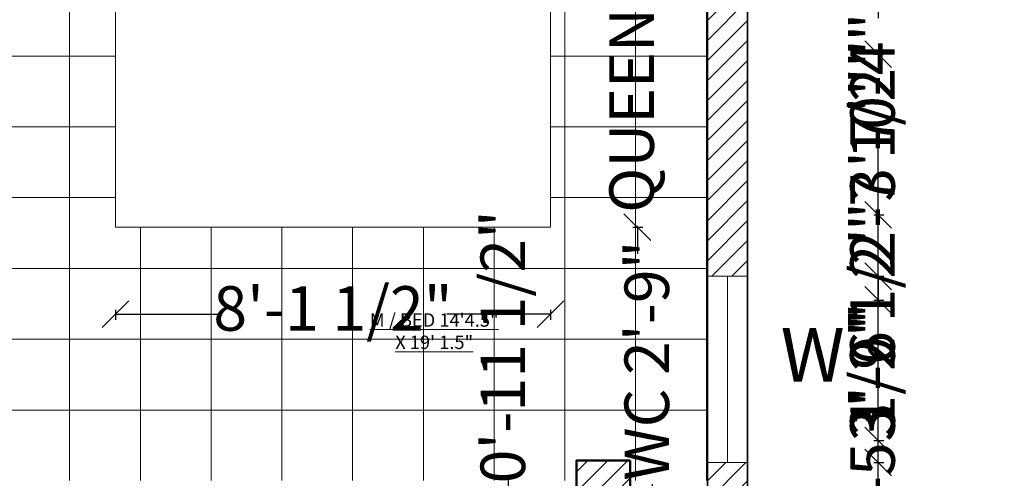
# Model space of a CAD drawing. Units: inches. Extents: x 2036 to 2670, y 319 to 920.
# Tile 14 of 15: x 2449 to 2670, y 620 to 723. Entities that reach past the tile are written whole.
import ezdxf

# ---------------------------------------------------------------- set-up
doc = ezdxf.new("R2010")
doc.units = ezdxf.units.IN
for name, color, linetype, lineweight in [('A-ANNO-DIMS', 2, 'Continuous', 18), ('A-ANNO-TEXT', 7, 'Continuous', 18), ('A-AREA-IDEN', 7, 'Continuous', 18), ('A-COLS', 7, 'Continuous', 50), ('A-FLOR-PATT', 8, 'Continuous', 9), ('A-FURN', 8, 'Continuous', 18), ('A-GLAZ', 4, 'Continuous', 18), ('A-WALL', 7, 'Continuous', 35)]:
    doc.layers.add(name, color=color, linetype=linetype, lineweight=lineweight)
doc.layers.add('A-COLS-PATT', color=240, linetype='Continuous', lineweight=13, true_color=0xed1f24)
doc.layers.add('A-WALL-PATT', color=52, linetype='Continuous', lineweight=13, true_color=0xc8c92d)
doc.styles.get("Standard").update_dxf_attribs({"font": 'arial.ttf'})
doc.dimstyles.new('ISO-25', dxfattribs={"dimtxt": 10, "dimasz": 6, "dimexe": 1.25, "dimexo": 0.625, "dimtad": 0, "dimdec": 1, "dimlunit": 3, "dimtxsty": 'Standard', "dimblk": 'OBLIQUE', "dimcen": 2.5, "dimclrd": 94, "dimclre": 94, "dimclrt": 1, "dimadec": 0, "dimazin": 0, "dimtfac": 1, "dimtdec": 1, "dimtmove": 0, "dimatfit": 3, "dimfxl": 1, "dimfxlon": 1, "dimarcsym": 0})

# ---------------------------------------------------------------- blocks, each defined once
blk = doc.blocks.new('Bed - Queen')
for p, q in [((0, -80.00003), (0, 0)), ((0, 0), (59.99999, 0)), ((59.99999, 0), (59.99999, -80.00003)), ((7.99999, -1.2), (28.79998, -1.2)), ((7.99999, -14.4), (7.99999, -1.2)), ((28.79998, -1.2), (28.79998, -14.4)), ((31.19999, -1.2), (51.99999, -1.2)), ((31.19999, -14.4), (31.19999, -1.2)), ((51.99999, -1.2), (51.99999, -16.4)), ((0, -14.4), (44.8, -14.4)), ((59.99999, -29.6), (44.8, -14.4)), ((44.8, -14.4), (44.8, -29.6)), ((44.8, -16.8), (0, -16.8)), ((51.99999, -16.4), (46.79936, -16.4)), ((44.8, -29.6), (59.99999, -29.6)), ((59.99999, -80.00003), (0, -80.00003))]:
    blk.add_line(p, q)
blk = doc.blocks.new('COL-9x12')
blk.add_lwpolyline([(9, 0), (0, 0), (0, 12), (9, 12)], close=True)
blk = doc.blocks.new('_Oblique')
at = {"color": 0, "linetype": 'ByBlock', "lineweight": -2}
blk.add_line((-0.5, -0.5), (0.5, 0.5), dxfattribs=at)
blk = doc.blocks.new('*D31')
at = {"layer": 'A-ANNO-DIMS', "color": 94, "lineweight": -2, "transparency": 16777216}
for p, q in [((2588.03, 806.13), (2588.03, 812.13)), ((2587.03, 806.13), (2589.28, 806.13)), ((2588.03, 806.13), (2588.03, 805.83)), ((2588.03, 676.01), (2588.03, 676.31)), ((2587.03, 676.01), (2589.28, 676.01)), ((2588.03, 676.01), (2588.03, 670.01))]:
    blk.add_line(p, q, dxfattribs=at)
at = {"layer": 'Defpoints', "color": 0, "transparency": 16777216}
for p in [(2568.52, 806.13), (2588.03, 806.13), (2568.52, 676.01)]:
    blk.add_point(p, dxfattribs=at)
at = {"layer": 'A-ANNO-DIMS', "color": 94, "lineweight": -2, "transparency": 16777216, "xscale": 6, "yscale": 6, "zscale": 6}
for p, rotation in [((2588.03, 806.13), 270), ((2588.03, 676.01), 90)]:
    blk.add_blockref('_Oblique', p, dxfattribs=dict(at, rotation=rotation))
at = {"layer": 'A-ANNO-DIMS', "color": 1, "transparency": 16777216, "insert": (2588.03, 741.07), "char_height": 10, "attachment_point": 5, "rotation": 90}
blk.add_mtext('QUEEN BED 10\'-10"', dxfattribs=at)
blk = doc.blocks.new('*D32')
at = {"layer": 'A-ANNO-DIMS', "color": 94, "lineweight": -2, "transparency": 16777216}
for p, q in [((2470.92, 657.49), (2470.92, 655.24)), ((2470.92, 656.49), (2494.15, 656.49)), ((2568.52, 656.49), (2545.29, 656.49)), ((2568.52, 657.49), (2568.52, 655.24))]:
    blk.add_line(p, q, dxfattribs=at)
at = {"layer": 'Defpoints', "color": 0, "transparency": 16777216}
for p in [(2470.92, 676.01), (2568.52, 676.01), (2568.52, 656.49)]:
    blk.add_point(p, dxfattribs=at)
at = {"layer": 'A-ANNO-DIMS', "color": 94, "lineweight": -2, "transparency": 16777216, "xscale": 6, "yscale": 6, "zscale": 6, "rotation": 180}
blk.add_blockref('_Oblique', (2470.92, 656.49), dxfattribs=at)
at = {"layer": 'A-ANNO-DIMS', "color": 94, "lineweight": -2, "transparency": 16777216, "xscale": 6, "yscale": 6, "zscale": 6}
blk.add_blockref('_Oblique', (2568.52, 656.49), dxfattribs=at)
at = {"layer": 'A-ANNO-DIMS', "color": 1, "transparency": 16777216, "insert": (2519.72, 656.49), "char_height": 10, "attachment_point": 5}
blk.add_mtext('8\'-1 1/2"', dxfattribs=at)
blk = doc.blocks.new('*D35')
at = {"layer": 'A-ANNO-DIMS', "color": 94, "lineweight": -2, "transparency": 16777216}
for p, q in [((2591.44, 612.38), (2591.44, 618.38)), ((2590.44, 612.38), (2592.69, 612.38)), ((2591.44, 579.34), (2591.44, 612.38)), ((2590.44, 579.34), (2592.69, 579.34))]:
    blk.add_line(p, q, dxfattribs=at)
at = {"layer": 'Defpoints', "color": 0, "transparency": 16777216}
for p in [(2586.48, 612.38), (2591.44, 612.38), (2586.48, 579.34)]:
    blk.add_point(p, dxfattribs=at)
at = {"layer": 'A-ANNO-DIMS', "color": 94, "lineweight": -2, "transparency": 16777216, "xscale": 6, "yscale": 6, "zscale": 6}
for p, rotation in [((2591.44, 612.38), 90), ((2591.44, 579.34), 270)]:
    blk.add_blockref('_Oblique', p, dxfattribs=dict(at, rotation=rotation))
at = {"layer": 'A-ANNO-DIMS', "color": 1, "transparency": 16777216, "insert": (2591.44, 646.08), "char_height": 10, "attachment_point": 5, "rotation": 90}
blk.add_mtext('WC 2\'-9"', dxfattribs=at)
blk = doc.blocks.new('*D37')
at = {"layer": 'A-ANNO-DIMS', "color": 94, "lineweight": -2, "transparency": 16777216}
for p, q in [((2541.16, 600.66), (2541.16, 598.41)), ((2541.16, 599.66), (2556.79, 599.66)), ((2556.79, 600.66), (2556.79, 598.41)), ((2556.79, 599.66), (2562.79, 599.66))]:
    blk.add_line(p, q, dxfattribs=at)
at = {"layer": 'Defpoints', "color": 0, "transparency": 16777216}
for p in [(2541.16, 602.01), (2556.79, 602.01), (2556.79, 599.66)]:
    blk.add_point(p, dxfattribs=at)
at = {"layer": 'A-ANNO-DIMS', "color": 94, "lineweight": -2, "transparency": 16777216, "xscale": 6, "yscale": 6, "zscale": 6, "rotation": 180}
blk.add_blockref('_Oblique', (2541.16, 599.66), dxfattribs=at)
at = {"layer": 'A-ANNO-DIMS', "color": 94, "lineweight": -2, "transparency": 16777216, "xscale": 6, "yscale": 6, "zscale": 6}
blk.add_blockref('_Oblique', (2556.79, 599.66), dxfattribs=at)
at = {"layer": 'A-ANNO-DIMS', "color": 1, "transparency": 16777216, "insert": (2617.95, 599.66), "char_height": 10, "attachment_point": 5}
blk.add_mtext('FAUCET 1\'-3 1/2"', dxfattribs=at)
blk = doc.blocks.new('*D38')
at = {"layer": 'A-ANNO-DIMS', "color": 94, "lineweight": -2, "transparency": 16777216}
for p, q in [((2559.13, 613.74), (2559.13, 619.74)), ((2558.13, 613.74), (2560.38, 613.74)), ((2559.13, 602.01), (2559.13, 613.74)), ((2558.13, 602.01), (2560.38, 602.01))]:
    blk.add_line(p, q, dxfattribs=at)
at = {"layer": 'Defpoints', "color": 0, "transparency": 16777216}
for p in [(2556.79, 613.74), (2559.13, 613.74), (2556.79, 602.01)]:
    blk.add_point(p, dxfattribs=at)
at = {"layer": 'A-ANNO-DIMS', "color": 94, "lineweight": -2, "transparency": 16777216, "xscale": 6, "yscale": 6, "zscale": 6}
for p, rotation in [((2559.13, 613.74), 90), ((2559.13, 602.01), 270)]:
    blk.add_blockref('_Oblique', p, dxfattribs=dict(at, rotation=rotation))
at = {"layer": 'A-ANNO-DIMS', "color": 1, "transparency": 16777216, "insert": (2559.13, 649.19), "char_height": 10, "attachment_point": 5, "rotation": 90}
blk.add_mtext('0\'-11 1/2"', dxfattribs=at)
blk = doc.blocks.new('*D46')
at = {"layer": 'A-ANNO-DIMS', "color": 94, "lineweight": -2, "transparency": 16777216}
for p, q in [((2642.09, 623.23), (2642.09, 629.23)), ((2641.09, 623.23), (2643.34, 623.23)), ((2642.09, 577.61), (2642.09, 623.23)), ((2641.09, 577.61), (2643.34, 577.61))]:
    blk.add_line(p, q, dxfattribs=at)
at = {"layer": 'Defpoints', "color": 0, "transparency": 16777216}
for p in [(2612.74, 623.23), (2642.09, 623.23), (2612.74, 577.61)]:
    blk.add_point(p, dxfattribs=at)
at = {"layer": 'A-ANNO-DIMS', "color": 94, "lineweight": -2, "transparency": 16777216, "xscale": 6, "yscale": 6, "zscale": 6}
for p, rotation in [((2642.09, 623.23), 90), ((2642.09, 577.61), 270)]:
    blk.add_blockref('_Oblique', p, dxfattribs=dict(at, rotation=rotation))
at = {"layer": 'A-ANNO-DIMS', "color": 1, "transparency": 16777216, "insert": (2642.09, 654.79), "char_height": 10, "attachment_point": 5, "rotation": 90}
blk.add_mtext('3\'-9 1/2"', dxfattribs=at)
blk = doc.blocks.new('*D47')
at = {"layer": 'A-ANNO-DIMS', "color": 94, "lineweight": -2, "transparency": 16777216}
for p, q in [((2641.09, 665), (2643.34, 665)), ((2642.09, 665), (2642.09, 658.03)), ((2642.09, 623.23), (2642.09, 630.2)), ((2641.09, 623.23), (2643.34, 623.23))]:
    blk.add_line(p, q, dxfattribs=at)
at = {"layer": 'Defpoints', "color": 0, "transparency": 16777216}
for p in [(2612.74, 665), (2642.09, 665), (2612.74, 623.23)]:
    blk.add_point(p, dxfattribs=at)
at = {"layer": 'A-ANNO-DIMS', "color": 94, "lineweight": -2, "transparency": 16777216, "xscale": 6, "yscale": 6, "zscale": 6}
for p, rotation in [((2642.09, 665), 90), ((2642.09, 623.23), 270)]:
    blk.add_blockref('_Oblique', p, dxfattribs=dict(at, rotation=rotation))
at = {"layer": 'A-ANNO-DIMS', "color": 1, "transparency": 16777216, "insert": (2642.09, 644.11), "char_height": 10, "attachment_point": 5, "rotation": 90}
blk.add_mtext('3\'-6"', dxfattribs=at)
blk = doc.blocks.new('*D48')
at = {"layer": 'A-ANNO-DIMS', "color": 94, "lineweight": -2, "transparency": 16777216}
for p, q in [((2641.09, 753.07), (2643.34, 753.07)), ((2642.09, 753.07), (2642.09, 722.91)), ((2642.09, 665), (2642.09, 695.16)), ((2641.09, 665), (2643.34, 665))]:
    blk.add_line(p, q, dxfattribs=at)
at = {"layer": 'Defpoints', "color": 0, "transparency": 16777216}
for p in [(2612.74, 753.07), (2642.09, 753.07), (2612.74, 665)]:
    blk.add_point(p, dxfattribs=at)
at = {"layer": 'A-ANNO-DIMS', "color": 94, "lineweight": -2, "transparency": 16777216, "xscale": 6, "yscale": 6, "zscale": 6}
for p, rotation in [((2642.09, 753.07), 90), ((2642.09, 665), 270)]:
    blk.add_blockref('_Oblique', p, dxfattribs=dict(at, rotation=rotation))
at = {"layer": 'A-ANNO-DIMS', "color": 1, "transparency": 16777216, "insert": (2642.09, 709.03), "char_height": 10, "attachment_point": 5, "rotation": 90}
blk.add_mtext('7\'-4"', dxfattribs=at)
blk = doc.blocks.new('*D56')
at = {"layer": 'A-ANNO-DIMS', "color": 94, "lineweight": -2, "transparency": 16777216}
for p, q in [((2642.09, 599.85), (2642.09, 605.85)), ((2641.09, 599.85), (2643.34, 599.85)), ((2642.09, 582.53), (2642.09, 599.85)), ((2641.09, 582.53), (2643.34, 582.53))]:
    blk.add_line(p, q, dxfattribs=at)
at = {"layer": 'Defpoints', "color": 0, "transparency": 16777216}
for p in [(2158.74, 599.85), (2642.09, 599.85), (2158.74, 582.53)]:
    blk.add_point(p, dxfattribs=at)
at = {"layer": 'A-ANNO-DIMS', "color": 94, "lineweight": -2, "transparency": 16777216, "xscale": 6, "yscale": 6, "zscale": 6}
for p, rotation in [((2642.09, 599.85), 90), ((2642.09, 582.53), 270)]:
    blk.add_blockref('_Oblique', p, dxfattribs=dict(at, rotation=rotation))
at = {"layer": 'A-ANNO-DIMS', "color": 1, "transparency": 16777216, "insert": (2642.09, 630.95), "char_height": 10, "attachment_point": 5, "rotation": 90}
blk.add_mtext('1\'-5 1/2"', dxfattribs=at)
blk = doc.blocks.new('*D57')
at = {"layer": 'A-ANNO-DIMS', "color": 94, "lineweight": -2, "transparency": 16777216}
for p, q in [((2642.09, 659.68), (2642.09, 665.68)), ((2641.09, 659.68), (2643.34, 659.68)), ((2642.09, 628.18), (2642.09, 659.68)), ((2641.09, 628.18), (2643.34, 628.18))]:
    blk.add_line(p, q, dxfattribs=at)
at = {"layer": 'Defpoints', "color": 0, "transparency": 16777216}
for p in [(2427.24, 659.68), (2642.09, 659.68), (2426.74, 628.18)]:
    blk.add_point(p, dxfattribs=at)
at = {"layer": 'A-ANNO-DIMS', "color": 94, "lineweight": -2, "transparency": 16777216, "xscale": 6, "yscale": 6, "zscale": 6}
for p, rotation in [((2642.09, 659.68), 90), ((2642.09, 628.18), 270)]:
    blk.add_blockref('_Oblique', p, dxfattribs=dict(at, rotation=rotation))
at = {"layer": 'A-ANNO-DIMS', "color": 1, "transparency": 16777216, "insert": (2642.09, 691.34), "char_height": 10, "attachment_point": 5, "rotation": 90}
blk.add_mtext('2\'-7 1/2"', dxfattribs=at)
blk = doc.blocks.new('*D59')
at = {"layer": 'A-ANNO-DIMS', "color": 94, "lineweight": -2, "transparency": 16777216}
for p, q in [((2641.09, 714.81), (2643.34, 714.81)), ((2642.09, 714.81), (2642.09, 710.72)), ((2642.09, 678.81), (2642.09, 682.89)), ((2641.09, 678.81), (2643.34, 678.81))]:
    blk.add_line(p, q, dxfattribs=at)
at = {"layer": 'Defpoints', "color": 0, "transparency": 16777216}
for p in [(2235.24, 714.81), (2642.09, 714.81), (2235.24, 678.81)]:
    blk.add_point(p, dxfattribs=at)
at = {"layer": 'A-ANNO-DIMS', "color": 94, "lineweight": -2, "transparency": 16777216, "xscale": 6, "yscale": 6, "zscale": 6}
for p, rotation in [((2642.09, 714.81), 90), ((2642.09, 678.81), 270)]:
    blk.add_blockref('_Oblique', p, dxfattribs=dict(at, rotation=rotation))
at = {"layer": 'A-ANNO-DIMS', "color": 1, "transparency": 16777216, "insert": (2642.09, 696.81), "char_height": 10, "attachment_point": 5, "rotation": 90}
blk.add_mtext('3\'-0"', dxfattribs=at)
blk = doc.blocks.new('*D60')
at = {"layer": 'A-ANNO-DIMS', "color": 94, "lineweight": -2, "transparency": 16777216}
for p, q in [((2051.39, 582.41), (2051.39, 588.41)), ((2052.39, 582.41), (2050.14, 582.41)), ((2051.39, 545.09), (2051.39, 582.41)), ((2052.39, 545.09), (2050.14, 545.09))]:
    blk.add_line(p, q, dxfattribs=at)
at = {"layer": 'Defpoints', "color": 0, "transparency": 16777216}
for p in [(2051.39, 582.41), (2515.24, 582.41), (2515.24, 545.09)]:
    blk.add_point(p, dxfattribs=at)
at = {"layer": 'A-ANNO-DIMS', "color": 94, "lineweight": -2, "transparency": 16777216, "xscale": 6, "yscale": 6, "zscale": 6}
for p, rotation in [((2051.39, 582.41), 90), ((2051.39, 545.09), 270)]:
    blk.add_blockref('_Oblique', p, dxfattribs=dict(at, rotation=rotation))
at = {"layer": 'A-ANNO-DIMS', "color": 1, "transparency": 16777216, "insert": (2051.39, 613.98), "char_height": 10, "attachment_point": 5, "rotation": 90}
blk.add_mtext('3\'-1 1/2"', dxfattribs=at)

msp = doc.modelspace()

# ---------------------------------------------------------------- hatches: boundary and pattern name
at = {"layer": 'A-COLS-PATT'}
h = msp.add_hatch(dxfattribs=at)
h.set_pattern_fill('ANSI31', color=256)
h.paths.add_polyline_path([(2089.74, 875.68), (2080.74, 875.68), (2080.74, 863.68), (2089.74, 863.68)])
h.paths.add_polyline_path([(2089.74, 821.68), (2080.74, 821.68), (2080.74, 809.68), (2089.74, 809.68)])
h.paths.add_polyline_path([(2089.74, 624.2), (2080.74, 624.2), (2080.74, 612.2), (2089.74, 612.2)])
h.paths.add_polyline_path([(2158.74, 506.68), (2149.74, 506.68), (2149.74, 494.68), (2158.74, 494.68)])
h.paths.add_polyline_path([(2158.74, 617.33), (2149.74, 617.33), (2149.74, 605.33), (2158.74, 605.33)])
h.paths.add_polyline_path([(2158.74, 736.18), (2149.74, 736.18), (2149.74, 724.18), (2158.74, 724.18)])
h.paths.add_polyline_path([(2158.74, 852.81), (2149.74, 852.81), (2149.74, 843.81), (2158.74, 843.81)])
h.paths.add_polyline_path([(2161.74, 852.81), (2158.74, 852.81), (2158.74, 843.81), (2161.74, 843.81)])
h.paths.add_polyline_path([(2295.21, 857.66), (2290.74, 857.66), (2290.74, 848.68), (2295.21, 848.68)])
h.paths.add_polyline_path([(2290.74, 857.66), (2283.21, 857.66), (2283.21, 848.66), (2290.74, 848.66)])
h.paths.add_polyline_path([(2443.62, 857.68), (2431.62, 857.68), (2431.62, 848.68), (2443.62, 848.68)])
h.paths.add_polyline_path([(2561.81, 857.68), (2549.81, 857.68), (2549.81, 848.68), (2561.81, 848.68)])
h.paths.add_polyline_path([(2295.24, 737.65), (2290.74, 737.65), (2290.74, 728.68), (2295.24, 728.68)])
h.paths.add_polyline_path([(2309.27, 612.12), (2297.27, 612.12), (2297.27, 603.12), (2309.27, 603.12)])
h.paths.add_polyline_path([(2282.24, 503.68), (2270.24, 503.68), (2270.24, 494.68), (2282.24, 494.68)])
h.paths.add_polyline_path([(2431.74, 746.09), (2427.24, 746.09), (2427.24, 737.09), (2431.74, 737.09)])
h.paths.add_polyline_path([(2439.24, 746.09), (2431.74, 746.09), (2431.74, 737.09), (2439.24, 737.09)])
h.paths.add_polyline_path([(2596.59, 736.59), (2584.59, 736.59), (2584.59, 727.59), (2596.59, 727.59)])
h.paths.add_polyline_path([(2586.39, 623.71), (2574.39, 623.71), (2574.39, 619.18), (2586.39, 619.18)])
h.paths.add_polyline_path([(2586.39, 619.18), (2574.39, 619.18), (2574.39, 614.71), (2586.39, 614.71)])
h.paths.add_polyline_path([(2438.74, 623.68), (2431.24, 623.68), (2431.24, 619.18), (2438.74, 619.18)])
h.paths.add_polyline_path([(2438.74, 619.18), (2431.24, 619.18), (2431.24, 614.68), (2438.74, 614.68)])
h.paths.add_polyline_path([(2431.24, 623.68), (2426.74, 623.68), (2426.74, 614.68), (2431.24, 614.68), (2431.24, 619.18)])
h.paths.add_polyline_path([(2527.24, 503.68), (2515.24, 503.68), (2515.24, 494.68), (2527.24, 494.68)])
h.paths.add_polyline_path([(2590.31, 503.68), (2578.31, 503.68), (2578.31, 494.68), (2590.31, 494.68)])
at = {"layer": 'A-FLOR-PATT'}
h = msp.add_hatch(dxfattribs=at)
h.set_pattern_fill('ANSI31', color=256, scale=5, angle=135)
h.paths.add_polyline_path([(2290.74, 659.68), (2158.74, 659.68), (2158.74, 582.53), (2158.74, 545.51), (2158.74, 503.68), (2426.74, 503.68), (2426.74, 614.68), (2426.74, 623.68), (2426.74, 628.18), (2431.24, 628.18), (2431.24, 623.68), (2438.74, 623.68), (2438.74, 619.18), (2574.39, 619.18), (2574.39, 623.71), (2586.39, 623.71), (2586.39, 619.18), (2603.74, 619.18), (2603.74, 824.68), (2431.74, 824.68), (2431.74, 746.09), (2439.24, 746.09), (2439.24, 737.09), (2431.74, 737.09), (2431.74, 659.68), (2427.24, 659.68), (2427.24, 739.48), (2383.24, 739.48), (2383.24, 804.68), (2339.24, 804.68), (2339.24, 749.08), (2295.24, 749.08), (2295.24, 737.65), (2295.27, 737.65), (2295.27, 728.65), (2295.21, 728.65, -0.586418), (2272.74, 728.68), (2272.74, 824.68), (2270.11, 824.68), (2270.11, 829.18), (2290.74, 829.18), (2290.74, 848.66), (2283.21, 848.66), (2283.21, 857.66), (2289.74, 857.66), (2289.74, 874.68), (2158.74, 874.68), (2158.74, 852.81), (2161.74, 852.81), (2161.74, 843.81), (2158.74, 843.81), (2158.74, 829.18), (2224.74, 829.18), (2224.74, 800.68), (2182.74, 800.68), (2182.74, 733.41), (2158.74, 733.41), (2158.74, 728.68), (2235.24, 728.68), (2235.24, 714.81), (2230.74, 714.81), (2230.74, 724.18), (2158.74, 724.18), (2158.74, 664.18), (2230.74, 664.18), (2230.74, 678.81), (2235.24, 678.81), (2235.24, 664.18), (2290.74, 664.18)])
h.paths.add_polyline_path([(2309.27, 612.12), (2309.27, 603.12), (2297.27, 603.12), (2297.27, 612.12)], flags=16)
h.paths.add_polyline_path([(2280.12, 639.11), (2280.26, 638.18, -0.414214), (2279.26, 637.18), (2278.76, 637.18), (2279.26, 633.18), (2277.76, 633.18), (2277.26, 637.18), (2269.76, 637.18), (2262.26, 637.18), (2261.76, 633.18), (2260.26, 633.18), (2260.76, 637.18), (2260.26, 637.18, -0.414214), (2259.26, 638.18), (2259.41, 639.11, -0.541164), (2257.76, 641.18), (2260.76, 652.18), (2261.45, 652.18), (2261.53, 652.68), (2262.76, 652.68), (2262.25, 655.24, 0.001913), (2261.76, 655.18), (2259.76, 658.18, -0.15), (2279.76, 658.18), (2277.76, 655.18, 0.001913), (2277.27, 655.24), (2276.76, 652.68), (2278, 652.68), (2278.07, 652.18), (2278.76, 652.18), (2281.76, 641.18, -0.541163)], flags=16)
h.paths.add_polyline_path([(2245.98, 639.11), (2246.13, 638.18, -0.414214), (2245.13, 637.18), (2244.63, 637.18), (2245.13, 633.18), (2243.63, 633.18), (2243.13, 637.18), (2235.63, 637.18), (2228.13, 637.18), (2227.63, 633.18), (2226.13, 633.18), (2226.63, 637.18), (2226.13, 637.18, -0.414214), (2225.13, 638.18), (2225.27, 639.11, -0.541164), (2223.63, 641.18), (2226.63, 652.18), (2227.32, 652.18), (2227.39, 652.68), (2228.63, 652.68), (2228.12, 655.24, 0.001913), (2227.63, 655.18), (2225.63, 658.18, -0.15), (2245.63, 658.18), (2243.63, 655.18, 0.001913), (2243.14, 655.24), (2242.63, 652.68), (2243.86, 652.68), (2243.94, 652.18), (2244.63, 652.18), (2247.63, 641.18, -0.541163)], flags=16)
h.paths.add_polyline_path([(2351.59, 515.15, -0.151948), (2279.59, 515.15), (2279.59, 537.68), (2273.59, 537.68), (2273.59, 511.68, 0.190476), (2357.59, 511.68), (2357.59, 537.68), (2351.59, 537.68)])
h.paths.add_polyline_path([(2327.59, 536.13), (2327.59, 517.07), (2303.59, 517.07), (2303.59, 536.13)], flags=16)
h.paths.add_polyline_path([(2213.4, 639.11), (2213.55, 638.18, -0.414214), (2212.55, 637.18), (2212.05, 637.18), (2212.55, 633.18), (2211.05, 633.18), (2210.55, 637.18), (2203.05, 637.18), (2195.55, 637.18), (2195.05, 633.18), (2193.55, 633.18), (2194.05, 637.18), (2193.55, 637.18, -0.414214), (2192.55, 638.18), (2192.69, 639.11, -0.541164), (2191.05, 641.18), (2194.05, 652.18), (2194.73, 652.18), (2194.81, 652.68), (2196.05, 652.68), (2195.53, 655.24, 0.001913), (2195.05, 655.18), (2193.05, 658.18, -0.15), (2213.05, 658.18), (2211.05, 655.18, 0.001913), (2210.56, 655.24), (2210.05, 652.68), (2211.28, 652.68), (2211.36, 652.18), (2212.05, 652.18), (2215.05, 641.18, -0.541163)], flags=16)
h.paths.add_polyline_path([(2368.58, 538.02), (2370.52, 538.02), (2371.17, 532.84), (2380.89, 532.84), (2390.6, 532.84), (2391.25, 538.02), (2393.2, 538.02), (2392.55, 532.84), (2380.89, 532.84), (2368.58, 532.84, 0.414214), (2367.28, 531.54), (2367.47, 530.34, -0.483352), (2369.23, 527.65), (2371.82, 513.4), (2370.12, 513.4), (2370.22, 512.75), (2391.56, 512.75), (2391.66, 513.4), (2389.96, 513.4), (2392.55, 527.65, -1.387427), (2396.43, 527.65), (2392.55, 513.4), (2391.66, 513.4), (2391.56, 512.75), (2389.31, 512.75), (2390, 509.37, 0.003796), (2391.25, 509.51), (2393.84, 505.63, -0.15), (2367.93, 505.63), (2370.52, 509.51, 0.003901), (2371.81, 509.36), (2372.47, 512.75), (2370.22, 512.75), (2370.12, 513.4), (2369.23, 513.4), (2365.34, 527.65, -0.541163), (2367.47, 530.34), (2367.28, 531.54, -0.414214), (2368.58, 532.84), (2369.23, 532.84)])
h.paths.add_polyline_path([(2266.74, 538.02), (2266.09, 532.84), (2254.43, 532.84), (2242.12, 532.84, 0.414214), (2240.83, 531.54), (2241.01, 530.34, -0.483352), (2242.77, 527.65), (2245.36, 513.4), (2243.66, 513.4), (2243.76, 512.75), (2265.1, 512.75), (2265.2, 513.4), (2263.5, 513.4), (2266.09, 527.65, -1.387427), (2269.98, 527.65), (2266.09, 513.4), (2265.2, 513.4), (2265.1, 512.75), (2262.85, 512.75), (2263.54, 509.37, 0.003796), (2264.79, 509.51), (2267.39, 505.63, -0.15), (2241.47, 505.63), (2244.07, 509.51, 0.003901), (2245.36, 509.36), (2246.01, 512.75), (2243.76, 512.75), (2243.66, 513.4), (2242.77, 513.4), (2238.88, 527.65, -0.541163), (2241.01, 530.34), (2240.83, 531.54, -0.414214), (2242.12, 532.84), (2242.77, 532.84), (2242.12, 538.02), (2244.07, 538.02), (2244.71, 532.84), (2254.43, 532.84), (2264.15, 532.84), (2264.79, 538.02)])
h.paths.add_polyline_path([(2185.24, 620.36), (2185.24, 618.86), (2181.24, 618.36), (2181.24, 610.86), (2181.24, 603.36), (2185.24, 602.86), (2185.24, 601.36), (2181.24, 601.86), (2181.24, 601.36, -0.414214), (2180.24, 600.36), (2179.31, 600.5, -0.541164), (2177.24, 598.86), (2166.24, 601.86), (2166.24, 602.54), (2165.74, 602.62), (2165.74, 603.86), (2163.18, 603.34, 0.001913), (2163.24, 602.86), (2160.24, 600.86, -0.15), (2160.24, 620.86), (2163.24, 618.86, 0.001913), (2163.18, 618.37), (2165.74, 617.86), (2165.74, 619.09), (2166.24, 619.17), (2166.24, 619.86), (2177.24, 622.86, -0.541163), (2179.31, 621.21), (2180.24, 621.36, -0.414214), (2181.24, 620.36), (2181.24, 619.86)])
h.paths.add_polyline_path([(2470.92, 676.01), (2470.92, 806.13), (2568.52, 806.13), (2568.52, 676.01)], flags=16)
h.paths.add_polyline_path([(2177.74, 677.49), (2161.9, 677.49), (2161.9, 705.85), (2177.74, 705.85)], flags=16)
h.paths.add_polyline_path([(2176.74, 678.49), (2162.9, 678.49), (2162.9, 704.85), (2176.74, 704.85)], flags=0)
h.paths.add_polyline_path([(2175.01, 686.48), (2172.93, 686.48), (2172.93, 690.63), (2170.86, 690.63), (2170.86, 686.48), (2164.63, 686.48), (2164.63, 688.56), (2166.71, 688.56), (2168.78, 688.56), (2168.78, 690.63), (2164.63, 690.63), (2164.63, 696.85), (2166.71, 696.85), (2166.71, 692.71), (2168.78, 692.71), (2168.78, 696.85), (2175.01, 696.85), (2175.01, 694.78), (2170.86, 694.78), (2170.86, 692.71), (2175.01, 692.71)], flags=0)
h.paths.add_polyline_path([(2543.79, 782.71), (2483.94, 782.71), (2483.94, 804.18), (2517.77, 804.18), (2517.77, 782.71), (2521.67, 782.71), (2521.67, 804.18), (2555.5, 804.18), (2555.5, 779.45), (2547.05, 779.45), (2568.52, 757.98), (2543.79, 757.98)], flags=0)
h.paths.add_polyline_path([(2584.59, 727.59), (2584.59, 736.59), (2596.59, 736.59), (2596.59, 727.59)], flags=16)
h.paths.add_polyline_path([(2520.45, 647.03), (2553.79, 647.03), (2553.79, 658.23), (2520.45, 658.23)], flags=24)
h.paths.add_polyline_path([(2299.53, 573.74), (2331.71, 573.74), (2331.71, 584.94), (2299.53, 584.94)], flags=24)
h.paths.add_polyline_path([(2191.59, 685.19), (2212.12, 685.19), (2212.12, 696.38), (2191.59, 696.38)], flags=24)
h.paths.add_polyline_path([(2353.9, 649.86), (2379.08, 649.86), (2379.08, 661.06), (2353.9, 661.06)], flags=24)
h.paths.add_polyline_path([(2214.61, 763.31), (2237.46, 763.31), (2237.46, 779.56), (2214.61, 779.56)], flags=24)
h.paths.add_polyline_path([(2225.09, 819.31), (2269.29, 819.31), (2269.29, 844.04), (2225.09, 844.04)], flags=24)
h.paths.add_polyline_path([(2204.06, 845.04), (2226.92, 845.04), (2226.92, 856.24), (2204.06, 856.24)], flags=24)
h = msp.add_hatch(dxfattribs=at)
h.set_pattern_fill('ANSI31', color=256, scale=5, angle=45)
h.paths.add_polyline_path([(2290.74, 659.68), (2158.74, 659.68), (2158.74, 582.53), (2158.74, 545.51), (2158.74, 503.68), (2426.74, 503.68), (2426.74, 614.68), (2426.74, 623.68), (2426.74, 628.18), (2431.24, 628.18), (2431.24, 623.68), (2438.74, 623.68), (2438.74, 619.18), (2574.39, 619.18), (2574.39, 623.71), (2586.39, 623.71), (2586.39, 619.18), (2603.74, 619.18), (2603.74, 824.68), (2431.74, 824.68), (2431.74, 746.09), (2439.24, 746.09), (2439.24, 737.09), (2431.74, 737.09), (2431.74, 659.68), (2427.24, 659.68), (2427.24, 739.48), (2383.24, 739.48), (2383.24, 804.68), (2339.24, 804.68), (2339.24, 749.08), (2295.24, 749.08), (2295.24, 737.65), (2295.27, 737.65), (2295.27, 728.65), (2295.21, 728.65, -0.586418), (2272.74, 728.68), (2272.74, 824.68), (2270.11, 824.68), (2270.11, 829.18), (2290.74, 829.18), (2290.74, 848.66), (2283.21, 848.66), (2283.21, 857.66), (2289.74, 857.66), (2289.74, 874.68), (2158.74, 874.68), (2158.74, 852.81), (2161.74, 852.81), (2161.74, 843.81), (2158.74, 843.81), (2158.74, 829.18), (2224.74, 829.18), (2224.74, 800.68), (2182.74, 800.68), (2182.74, 733.41), (2158.74, 733.41), (2158.74, 728.68), (2235.24, 728.68), (2235.24, 714.81), (2230.74, 714.81), (2230.74, 724.18), (2158.74, 724.18), (2158.74, 664.18), (2230.74, 664.18), (2230.74, 678.81), (2235.24, 678.81), (2235.24, 664.18), (2290.74, 664.18)])
h.paths.add_polyline_path([(2309.27, 612.12), (2309.27, 603.12), (2297.27, 603.12), (2297.27, 612.12)], flags=16)
h.paths.add_polyline_path([(2280.12, 639.11), (2280.26, 638.18, -0.414214), (2279.26, 637.18), (2278.76, 637.18), (2279.26, 633.18), (2277.76, 633.18), (2277.26, 637.18), (2269.76, 637.18), (2262.26, 637.18), (2261.76, 633.18), (2260.26, 633.18), (2260.76, 637.18), (2260.26, 637.18, -0.414214), (2259.26, 638.18), (2259.41, 639.11, -0.541164), (2257.76, 641.18), (2260.76, 652.18), (2261.45, 652.18), (2261.53, 652.68), (2262.76, 652.68), (2262.25, 655.24, 0.001913), (2261.76, 655.18), (2259.76, 658.18, -0.15), (2279.76, 658.18), (2277.76, 655.18, 0.001913), (2277.27, 655.24), (2276.76, 652.68), (2278, 652.68), (2278.07, 652.18), (2278.76, 652.18), (2281.76, 641.18, -0.541163)], flags=16)
h.paths.add_polyline_path([(2245.98, 639.11), (2246.13, 638.18, -0.414214), (2245.13, 637.18), (2244.63, 637.18), (2245.13, 633.18), (2243.63, 633.18), (2243.13, 637.18), (2235.63, 637.18), (2228.13, 637.18), (2227.63, 633.18), (2226.13, 633.18), (2226.63, 637.18), (2226.13, 637.18, -0.414214), (2225.13, 638.18), (2225.27, 639.11, -0.541164), (2223.63, 641.18), (2226.63, 652.18), (2227.32, 652.18), (2227.39, 652.68), (2228.63, 652.68), (2228.12, 655.24, 0.001913), (2227.63, 655.18), (2225.63, 658.18, -0.15), (2245.63, 658.18), (2243.63, 655.18, 0.001913), (2243.14, 655.24), (2242.63, 652.68), (2243.86, 652.68), (2243.94, 652.18), (2244.63, 652.18), (2247.63, 641.18, -0.541163)], flags=16)
h.paths.add_polyline_path([(2351.59, 537.68), (2351.59, 515.15, -0.151948), (2279.59, 515.15), (2279.59, 537.68), (2273.59, 537.68), (2273.59, 511.68, 0.190476), (2357.59, 511.68), (2357.59, 537.68)])
h.paths.add_polyline_path([(2368.58, 538.02), (2370.52, 538.02), (2371.17, 532.84), (2380.89, 532.84), (2390.6, 532.84), (2391.25, 538.02), (2393.2, 538.02), (2392.55, 532.84), (2380.89, 532.84), (2368.58, 532.84, 0.414214), (2367.28, 531.54), (2367.47, 530.34, -0.483352), (2369.23, 527.65), (2371.82, 513.4), (2370.12, 513.4), (2370.22, 512.75), (2391.56, 512.75), (2391.66, 513.4), (2389.96, 513.4), (2392.55, 527.65, -1.387427), (2396.43, 527.65), (2392.55, 513.4), (2391.66, 513.4), (2391.56, 512.75), (2389.31, 512.75), (2390, 509.37, 0.003796), (2391.25, 509.51), (2393.84, 505.63, -0.15), (2367.93, 505.63), (2370.52, 509.51, 0.003901), (2371.81, 509.36), (2372.47, 512.75), (2370.22, 512.75), (2370.12, 513.4), (2369.23, 513.4), (2365.34, 527.65, -0.541163), (2367.47, 530.34), (2367.28, 531.54, -0.414214), (2368.58, 532.84), (2369.23, 532.84)])
h.paths.add_polyline_path([(2327.59, 536.13), (2327.59, 517.07), (2303.59, 517.07), (2303.59, 536.13)], flags=16)
h.paths.add_polyline_path([(2470.92, 676.01), (2470.92, 806.13), (2568.52, 806.13), (2568.52, 676.01)], flags=16)
h.paths.add_polyline_path([(2266.74, 538.02), (2266.09, 532.84), (2254.43, 532.84), (2242.12, 532.84, 0.414214), (2240.83, 531.54), (2241.01, 530.34, -0.483352), (2242.77, 527.65), (2245.36, 513.4), (2243.66, 513.4), (2243.76, 512.75), (2265.1, 512.75), (2265.2, 513.4), (2263.5, 513.4), (2266.09, 527.65, -1.387427), (2269.98, 527.65), (2266.09, 513.4), (2265.2, 513.4), (2265.1, 512.75), (2262.85, 512.75), (2263.54, 509.37, 0.003796), (2264.79, 509.51), (2267.39, 505.63, -0.15), (2241.47, 505.63), (2244.07, 509.51, 0.003901), (2245.36, 509.36), (2246.01, 512.75), (2243.76, 512.75), (2243.66, 513.4), (2242.77, 513.4), (2238.88, 527.65, -0.541163), (2241.01, 530.34), (2240.83, 531.54, -0.414214), (2242.12, 532.84), (2242.77, 532.84), (2242.12, 538.02), (2244.07, 538.02), (2244.71, 532.84), (2254.43, 532.84), (2264.15, 532.84), (2264.79, 538.02)])
h.paths.add_polyline_path([(2213.4, 639.11), (2213.55, 638.18, -0.414214), (2212.55, 637.18), (2212.05, 637.18), (2212.55, 633.18), (2211.05, 633.18), (2210.55, 637.18), (2203.05, 637.18), (2195.55, 637.18), (2195.05, 633.18), (2193.55, 633.18), (2194.05, 637.18), (2193.55, 637.18, -0.414214), (2192.55, 638.18), (2192.69, 639.11, -0.541164), (2191.05, 641.18), (2194.05, 652.18), (2194.73, 652.18), (2194.81, 652.68), (2196.05, 652.68), (2195.53, 655.24, 0.001913), (2195.05, 655.18), (2193.05, 658.18, -0.15), (2213.05, 658.18), (2211.05, 655.18, 0.001913), (2210.56, 655.24), (2210.05, 652.68), (2211.28, 652.68), (2211.36, 652.18), (2212.05, 652.18), (2215.05, 641.18, -0.541163)], flags=16)
h.paths.add_polyline_path([(2185.24, 620.36), (2185.24, 618.86), (2181.24, 618.36), (2181.24, 610.86), (2181.24, 603.36), (2185.24, 602.86), (2185.24, 601.36), (2181.24, 601.86), (2181.24, 601.36, -0.414214), (2180.24, 600.36), (2179.31, 600.5, -0.541164), (2177.24, 598.86), (2166.24, 601.86), (2166.24, 602.54), (2165.74, 602.62), (2165.74, 603.86), (2163.18, 603.34, 0.001913), (2163.24, 602.86), (2160.24, 600.86, -0.15), (2160.24, 620.86), (2163.24, 618.86, 0.001913), (2163.18, 618.37), (2165.74, 617.86), (2165.74, 619.09), (2166.24, 619.17), (2166.24, 619.86), (2177.24, 622.86, -0.541163), (2179.31, 621.21), (2180.24, 621.36, -0.414214), (2181.24, 620.36), (2181.24, 619.86)])
h.paths.add_polyline_path([(2177.74, 677.49), (2161.9, 677.49), (2161.9, 705.85), (2177.74, 705.85)], flags=16)
h.paths.add_polyline_path([(2176.74, 678.49), (2162.9, 678.49), (2162.9, 704.85), (2176.74, 704.85)], flags=0)
h.paths.add_polyline_path([(2175.01, 686.48), (2172.93, 686.48), (2172.93, 690.63), (2170.86, 690.63), (2170.86, 686.48), (2164.63, 686.48), (2164.63, 688.56), (2166.71, 688.56), (2168.78, 688.56), (2168.78, 690.63), (2164.63, 690.63), (2164.63, 696.85), (2166.71, 696.85), (2166.71, 692.71), (2168.78, 692.71), (2168.78, 696.85), (2175.01, 696.85), (2175.01, 694.78), (2170.86, 694.78), (2170.86, 692.71), (2175.01, 692.71)], flags=0)
h.paths.add_polyline_path([(2543.79, 782.71), (2483.94, 782.71), (2483.94, 804.18), (2517.77, 804.18), (2517.77, 782.71), (2521.67, 782.71), (2521.67, 804.18), (2555.5, 804.18), (2555.5, 779.45), (2547.05, 779.45), (2568.52, 757.98), (2543.79, 757.98)], flags=0)
h.paths.add_polyline_path([(2584.59, 727.59), (2584.59, 736.59), (2596.59, 736.59), (2596.59, 727.59)], flags=16)
h.paths.add_polyline_path([(2520.45, 647.03), (2553.79, 647.03), (2553.79, 658.23), (2520.45, 658.23)], flags=24)
h.paths.add_polyline_path([(2299.53, 573.74), (2331.71, 573.74), (2331.71, 584.94), (2299.53, 584.94)], flags=24)
h.paths.add_polyline_path([(2191.59, 685.19), (2212.12, 685.19), (2212.12, 696.38), (2191.59, 696.38)], flags=24)
h.paths.add_polyline_path([(2353.9, 649.86), (2379.08, 649.86), (2379.08, 661.06), (2353.9, 661.06)], flags=24)
h.paths.add_polyline_path([(2214.61, 763.31), (2237.46, 763.31), (2237.46, 779.56), (2214.61, 779.56)], flags=24)
h.paths.add_polyline_path([(2225.09, 819.31), (2269.29, 819.31), (2269.29, 844.04), (2225.09, 844.04)], flags=24)
h.paths.add_polyline_path([(2204.06, 845.04), (2226.92, 845.04), (2226.92, 856.24), (2204.06, 856.24)], flags=24)
h = msp.add_hatch(dxfattribs=at)
h.set_pattern_fill('ANSI31', color=256, scale=3, angle=135)
h.paths.add_polyline_path([(2149.74, 582.53), (2149.74, 707.68), (2120.74, 707.68), (2120.74, 599.68, -1), (2118.74, 599.68), (2085.24, 599.68), (2085.24, 506.68), (2089.74, 506.68), (2089.74, 494.68), (2085.24, 494.68), (2085.24, 469.18), (2608.24, 469.18), (2608.24, 494.68), (2149.74, 494.68), (2149.74, 506.68), (2149.74, 545.51)])
h.paths.add_polyline_path([(2143.58, 686.71), (2149.03, 686.71), (2149.03, 692.89), (2143.58, 692.89)], flags=24)
h.paths.add_polyline_path([(2125.99, 700.31), (2133.31, 700.31), (2133.31, 706.49), (2125.99, 706.49)], flags=24)
at = {"layer": 'A-WALL-PATT'}
h = msp.add_hatch(dxfattribs=at)
h.set_pattern_fill('ANSI31', color=256)
h.paths.add_polyline_path([(2561.81, 857.68), (2561.81, 848.68), (2603.74, 848.68), (2603.74, 798.38), (2612.74, 798.38), (2612.74, 857.68)])
h.paths.add_polyline_path([(2603.74, 665), (2612.74, 665), (2612.74, 753.07), (2603.74, 753.07)])
h.paths.add_polyline_path([(2612.74, 623.23), (2603.74, 623.23), (2603.74, 614.68), (2603.74, 577.61), (2612.74, 577.61)])
h.paths.add_polyline_path([(2612.74, 553.61), (2603.74, 553.61), (2603.74, 503.68), (2612.74, 503.68)])

# ---------------------------------------------------------------- linework, layer by layer
at = {"layer": 'A-GLAZ'}
for p, q in [((2603.74, 665), (2612.74, 665)), ((2608.24, 623.23), (2608.24, 665)), ((2603.74, 623.23), (2612.74, 623.23))]:
    msp.add_line(p, q, dxfattribs=at)
at = {"layer": 'A-WALL'}
for p, q in [((2612.74, 494.13), (2612.74, 857.68)), ((2603.74, 614.68), (2603.74, 848.68))]:
    msp.add_line(p, q, dxfattribs=at)

# ---------------------------------------------------------------- block references
at = {"layer": 'A-COLS', "rotation": 89.99999999999737}
msp.add_blockref('COL-9x12', (2586.39, 614.71), dxfattribs=at)
at = {"layer": 'A-FURN', "xscale": 1.626514147143349, "yscale": 1.626514147143349, "zscale": 1.626514147143349}
msp.add_blockref('Bed - Queen', (2470.92, 806.13), dxfattribs=at)

# ---------------------------------------------------------------- texts
at = {"layer": 'A-ANNO-TEXT', "insert": (2620.18, 653.39), "char_height": 12, "attachment_point": 1}
msp.add_mtext_dynamic_manual_height_columns('W', width=27.6972, gutter_width=12.5, heights=[0], dxfattribs=at)
at = {"layer": 'A-AREA-IDEN', "insert": (2542.45, 656.69), "char_height": 3, "width": 31.9989, "attachment_point": 2}
msp.add_mtext('\\LM / BED\\l \\L14\'4.5" X 19\' 1.5"\\l', dxfattribs=at)

# ---------------------------------------------------------------- dimensions: what is measured, and where the dimension line sits
at = {"layer": 'A-ANNO-DIMS'}
for base, p1, p2, text, picture, middle in [((2588.03, 806.13), (2568.52, 676.01), (2568.52, 806.13), 'QUEEN BED <>', '*D31', (2588.03, 741.07)), ((2591.44, 612.38), (2586.48, 579.34), (2586.48, 612.38), 'WC <>', '*D35', (2591.44, 646.08))]:
    dim = msp.add_linear_dim(base=base, p1=p1, p2=p2, angle=90, text=text, dimstyle='ISO-25', override={"dimdec": 1, "dimlfac": 1, "dimrnd": 0, "dimzin": 1, "dimdsep": 46, "dimlunit": 4, "dimfrac": 2}, dxfattribs=at)
    dim.commit()
    dim.dimension.update_dxf_attribs({"geometry": picture, "text_midpoint": middle})
for base, p1, p2, picture, middle in [((2642.09, 753.07), (2612.74, 665), (2612.74, 753.07), '*D48', (2642.09, 709.03)), ((2642.09, 714.81), (2235.24, 678.81), (2235.24, 714.81), '*D59', (2642.09, 696.81)), ((2642.09, 659.68), (2426.74, 628.18), (2427.24, 659.68), '*D57', (2642.09, 691.34)), ((2559.13, 613.74), (2556.79, 602.01), (2556.79, 613.74), '*D38', (2559.13, 649.19)), ((2642.09, 623.23), (2612.74, 577.61), (2612.74, 623.23), '*D46', (2642.09, 654.79)), ((2642.09, 665), (2612.74, 623.23), (2612.74, 665), '*D47', (2642.09, 644.11)), ((2642.09, 599.85), (2158.74, 582.53), (2158.74, 599.85), '*D56', (2642.09, 630.95)), ((2051.39, 582.41), (2515.24, 545.09), (2515.24, 582.41), '*D60', (2051.39, 613.98))]:
    dim = msp.add_linear_dim(base=base, p1=p1, p2=p2, angle=90, dimstyle='ISO-25', override={"dimdec": 1, "dimlfac": 1, "dimrnd": 0, "dimzin": 1, "dimdsep": 46, "dimlunit": 4, "dimfrac": 2}, dxfattribs=at)
    dim.commit()
    dim.dimension.update_dxf_attribs({"geometry": picture, "text_midpoint": middle})
dim = msp.add_linear_dim(base=(2568.52, 656.49), p1=(2470.92, 676.01), p2=(2568.52, 676.01), dimstyle='ISO-25', override={"dimdec": 1, "dimlfac": 1, "dimrnd": 0, "dimzin": 1, "dimdsep": 46, "dimlunit": 4, "dimfrac": 2}, dxfattribs=at)
dim.commit()
dim.dimension.update_dxf_attribs({"geometry": '*D32', "text_midpoint": (2519.72, 656.49)})
dim = msp.add_linear_dim(base=(2556.79, 599.66), p1=(2541.16, 602.01), p2=(2556.79, 602.01), text='FAUCET <>', dimstyle='ISO-25', override={"dimdec": 1, "dimlfac": 1, "dimrnd": 0, "dimzin": 1, "dimdsep": 46, "dimlunit": 4, "dimfrac": 2}, dxfattribs=at)
dim.commit()
dim.dimension.update_dxf_attribs({"geometry": '*D37', "text_midpoint": (2617.95, 599.66)})

doc.saveas('drawing.dxf')
